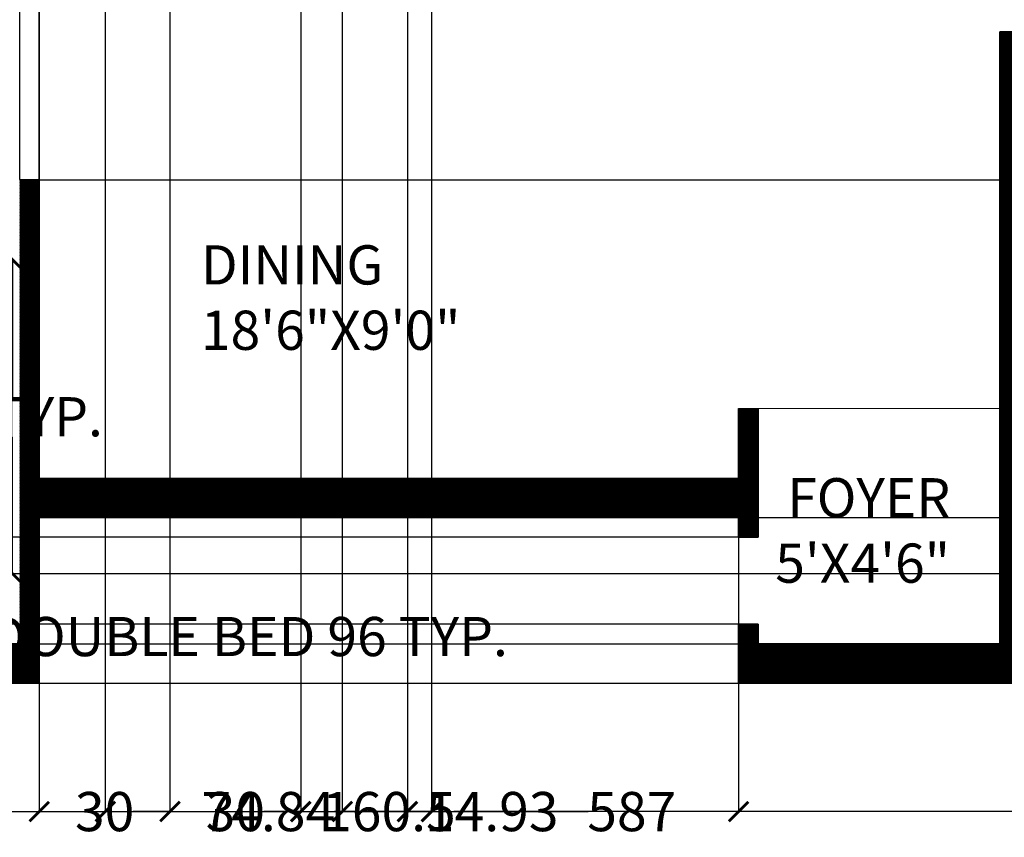
# Model space of a CAD drawing. Units: inches. Extents: x -9 to 675, y 146 to 566.
# Tile 2 of 4: x 192 to 418, y 146 to 334. Entities that reach past the tile are written whole.
import ezdxf

# ---------------------------------------------------------------- set-up
doc = ezdxf.new("R2010")
doc.units = ezdxf.units.IN
doc.header["$MEASUREMENT"] = 0
for name, color, linetype, lineweight in [('A-ANNO-DIMS', 2, 'Continuous', 18), ('A-AREA-IDEN', 7, 'Continuous', 18), ('A-FLOR-TRNS', 8, 'Continuous', 13), ('A-WALL', 7, 'Continuous', 35), ('A-WALL-PATT', 252, 'Continuous', 13)]:
    doc.layers.add(name, color=color, linetype=linetype, lineweight=lineweight)
doc.styles.get("Standard").update_dxf_attribs({"font": 'arial.ttf'})
doc.dimstyles.get("Standard").update_dxf_attribs({"dimtxt": 9, "dimasz": 4.5, "dimexe": 0.18, "dimexo": 0.0625, "dimgap": 0.09, "dimtad": 0, "dimtih": 1, "dimtoh": 1, "dimdec": 1, "dimzin": 0, "dimdsep": 46, "dimlunit": 4, "dimtxsty": 'Standard', "dimblk": 'ARCHTICK', "dimcen": 0.09, "dimadec": 0, "dimazin": 0, "dimtfac": 1, "dimtdec": 1, "dimtofl": 0, "dimtmove": 0, "dimatfit": 3, "dimfxl": 1, "dimtolj": 1, "dimtzin": 0, "dimarcsym": 0})

# ---------------------------------------------------------------- blocks, each defined once
blk = doc.blocks.new('_ArchTick')
at = {"color": 0, "linetype": 'ByBlock', "const_width": 0.15}
blk.add_lwpolyline([(-0.5, -0.5), (0.5, 0.5)], dxfattribs=at)
blk = doc.blocks.new('*D4')
at = {"layer": 'A-ANNO-DIMS', "color": 0, "lineweight": -2, "transparency": 16777216}
for p, q in [((80.28, 206.51), (80.28, 192)), ((176.28, 206.51), (176.28, 192)), ((80.28, 192.18), (176.28, 192.18)), ((176.28, 192.18), (180.78, 192.18))]:
    blk.add_line(p, q, dxfattribs=at)
at = {"layer": 'Defpoints', "color": 0, "transparency": 16777216}
for p in [(80.28, 206.58), (176.28, 206.58), (176.28, 192.18)]:
    blk.add_point(p, dxfattribs=at)
at = {"layer": 'A-ANNO-DIMS', "color": 0, "lineweight": -2, "transparency": 16777216, "xscale": 4.5, "yscale": 4.5, "zscale": 4.5, "rotation": 180}
blk.add_blockref('_ArchTick', (80.28, 192.18), dxfattribs=at)
at = {"layer": 'A-ANNO-DIMS', "color": 0, "lineweight": -2, "transparency": 16777216, "xscale": 4.5, "yscale": 4.5, "zscale": 4.5}
blk.add_blockref('_ArchTick', (176.28, 192.18), dxfattribs=at)
at = {"layer": 'A-ANNO-DIMS', "color": 0, "transparency": 16777216, "insert": (244.83, 192.18), "char_height": 9, "attachment_point": 5}
blk.add_mtext('\\A1;DOUBLE BED 96 TYP.', dxfattribs=at)
blk = doc.blocks.new('*D5')
at = {"layer": 'A-ANNO-DIMS', "color": 0, "lineweight": -2, "transparency": 16777216}
for p, q in [((176.35, 278.67), (190.86, 278.67)), ((190.68, 278.67), (190.68, 247.24)), ((190.68, 206.58), (190.68, 238.01)), ((176.35, 206.58), (190.86, 206.58))]:
    blk.add_line(p, q, dxfattribs=at)
at = {"layer": 'Defpoints', "color": 0, "transparency": 16777216}
for p in [(176.28, 278.67), (190.68, 278.67), (176.28, 206.58)]:
    blk.add_point(p, dxfattribs=at)
at = {"layer": 'A-ANNO-DIMS', "color": 0, "lineweight": -2, "transparency": 16777216, "xscale": 4.5, "yscale": 4.5, "zscale": 4.5}
for p, rotation in [((190.68, 278.67), 90), ((190.68, 206.58), 270)]:
    blk.add_blockref('_ArchTick', p, dxfattribs=dict(at, rotation=rotation))
at = {"layer": 'A-ANNO-DIMS', "color": 0, "transparency": 16777216, "insert": (190.68, 242.63), "char_height": 9, "attachment_point": 5}
blk.add_mtext('\\A1;72 TYP.', dxfattribs=at)
blk = doc.blocks.new('*D8')
at = {"layer": 'A-ANNO-DIMS', "color": 0, "lineweight": -2, "transparency": 16777216}
for p, q in [((626.3, 217.45), (626.3, 151.83)), ((39.3, 181.45), (39.3, 151.83)), ((39.3, 152.01), (322.77, 152.01)), ((626.3, 152.01), (342.83, 152.01))]:
    blk.add_line(p, q, dxfattribs=at)
at = {"layer": 'Defpoints', "color": 0, "transparency": 16777216}
for p in [(626.3, 217.51), (39.3, 181.51), (626.3, 152.01)]:
    blk.add_point(p, dxfattribs=at)
at = {"layer": 'A-ANNO-DIMS', "color": 0, "lineweight": -2, "transparency": 16777216, "xscale": 4.5, "yscale": 4.5, "zscale": 4.5, "rotation": 180}
blk.add_blockref('_ArchTick', (39.3, 152.01), dxfattribs=at)
at = {"layer": 'A-ANNO-DIMS', "color": 0, "lineweight": -2, "transparency": 16777216, "xscale": 4.5, "yscale": 4.5, "zscale": 4.5}
blk.add_blockref('_ArchTick', (626.3, 152.01), dxfattribs=at)
at = {"layer": 'A-ANNO-DIMS', "color": 0, "transparency": 16777216, "insert": (332.8, 152.01), "char_height": 9, "attachment_point": 5}
blk.add_mtext('\\A1;587', dxfattribs=at)
blk = doc.blocks.new('*D20')
at = {"layer": 'A-ANNO-DIMS', "color": 0, "lineweight": -2, "transparency": 16777216}
for p, q in [((196.8, 219.43), (196.8, 151.83)), ((357.3, 219.43), (357.3, 151.83)), ((196.8, 152.01), (262.17, 152.01)), ((357.3, 152.01), (291.94, 152.01))]:
    blk.add_line(p, q, dxfattribs=at)
at = {"layer": 'Defpoints', "color": 0, "transparency": 16777216}
for p in [(196.8, 219.49), (357.3, 219.49), (357.3, 152.01)]:
    blk.add_point(p, dxfattribs=at)
at = {"layer": 'A-ANNO-DIMS', "color": 0, "lineweight": -2, "transparency": 16777216, "xscale": 4.5, "yscale": 4.5, "zscale": 4.5, "rotation": 180}
blk.add_blockref('_ArchTick', (196.8, 152.01), dxfattribs=at)
at = {"layer": 'A-ANNO-DIMS', "color": 0, "lineweight": -2, "transparency": 16777216, "xscale": 4.5, "yscale": 4.5, "zscale": 4.5}
blk.add_blockref('_ArchTick', (357.3, 152.01), dxfattribs=at)
at = {"layer": 'A-ANNO-DIMS', "color": 0, "transparency": 16777216, "insert": (277.05, 152.01), "char_height": 9, "attachment_point": 5}
blk.add_mtext('\\A1;160.5', dxfattribs=at)
blk = doc.blocks.new('*D22')
at = {"layer": 'A-ANNO-DIMS', "color": 0, "lineweight": -2, "transparency": 16777216}
for p, q in [((196.87, 219.49), (655.98, 219.49)), ((655.8, 219.49), (655.8, 205.19)), ((655.8, 181.51), (655.8, 195.81)), ((196.87, 181.51), (655.98, 181.51))]:
    blk.add_line(p, q, dxfattribs=at)
at = {"layer": 'Defpoints', "color": 0, "transparency": 16777216}
for p in [(196.8, 219.49), (655.8, 219.49), (196.8, 181.51)]:
    blk.add_point(p, dxfattribs=at)
at = {"layer": 'A-ANNO-DIMS', "color": 0, "lineweight": -2, "transparency": 16777216, "xscale": 4.5, "yscale": 4.5, "zscale": 4.5}
for p, rotation in [((655.8, 219.49), 90), ((655.8, 181.51), 270)]:
    blk.add_blockref('_ArchTick', p, dxfattribs=dict(at, rotation=rotation))
at = {"layer": 'A-ANNO-DIMS', "color": 0, "transparency": 16777216, "insert": (655.8, 200.5), "char_height": 9, "attachment_point": 5}
blk.add_mtext('\\A1;37.98', dxfattribs=at)
blk = doc.blocks.new('*D26')
at = {"layer": 'A-ANNO-DIMS', "color": 0, "lineweight": -2, "transparency": 16777216}
for p, q in [((211.96, 521.95), (211.96, 151.83)), ((286.8, 521.95), (286.8, 151.83)), ((211.96, 152.01), (234.16, 152.01)), ((286.8, 152.01), (264.6, 152.01))]:
    blk.add_line(p, q, dxfattribs=at)
at = {"layer": 'Defpoints', "color": 0, "transparency": 16777216}
for p in [(211.96, 522.01), (286.8, 522.01), (286.8, 152.01)]:
    blk.add_point(p, dxfattribs=at)
at = {"layer": 'A-ANNO-DIMS', "color": 0, "lineweight": -2, "transparency": 16777216, "xscale": 4.5, "yscale": 4.5, "zscale": 4.5, "rotation": 180}
blk.add_blockref('_ArchTick', (211.96, 152.01), dxfattribs=at)
at = {"layer": 'A-ANNO-DIMS', "color": 0, "lineweight": -2, "transparency": 16777216, "xscale": 4.5, "yscale": 4.5, "zscale": 4.5}
blk.add_blockref('_ArchTick', (286.8, 152.01), dxfattribs=at)
at = {"layer": 'A-ANNO-DIMS', "color": 0, "transparency": 16777216, "insert": (249.38, 152.01), "char_height": 9, "attachment_point": 5}
blk.add_mtext('\\A1;74.84', dxfattribs=at)
blk = doc.blocks.new('*D28')
at = {"layer": 'A-ANNO-DIMS', "color": 0, "lineweight": -2, "transparency": 16777216}
for p, q in [((196.8, 469.45), (196.8, 151.83)), ((226.8, 469.45), (226.8, 151.83)), ((196.8, 152.01), (205.28, 152.01)), ((226.8, 152.01), (218.32, 152.01))]:
    blk.add_line(p, q, dxfattribs=at)
at = {"layer": 'Defpoints', "color": 0, "transparency": 16777216}
for p in [(196.8, 469.51), (226.8, 469.51), (226.8, 152.01)]:
    blk.add_point(p, dxfattribs=at)
at = {"layer": 'A-ANNO-DIMS', "color": 0, "lineweight": -2, "transparency": 16777216, "xscale": 4.5, "yscale": 4.5, "zscale": 4.5, "rotation": 180}
blk.add_blockref('_ArchTick', (196.8, 152.01), dxfattribs=at)
at = {"layer": 'A-ANNO-DIMS', "color": 0, "lineweight": -2, "transparency": 16777216, "xscale": 4.5, "yscale": 4.5, "zscale": 4.5}
blk.add_blockref('_ArchTick', (226.8, 152.01), dxfattribs=at)
at = {"layer": 'A-ANNO-DIMS', "color": 0, "transparency": 16777216, "insert": (211.8, 152.01), "char_height": 9, "attachment_point": 5}
blk.add_mtext('\\A1;30', dxfattribs=at)
blk = doc.blocks.new('*D29')
at = {"layer": 'A-ANNO-DIMS', "color": 0, "lineweight": -2, "transparency": 16777216}
for p, q in [((226.8, 469.45), (226.8, 151.83)), ((256.8, 469.45), (256.8, 151.83)), ((226.8, 152.01), (235.28, 152.01)), ((256.8, 152.01), (248.32, 152.01))]:
    blk.add_line(p, q, dxfattribs=at)
at = {"layer": 'Defpoints', "color": 0, "transparency": 16777216}
for p in [(226.8, 469.51), (256.8, 469.51), (256.8, 152.01)]:
    blk.add_point(p, dxfattribs=at)
at = {"layer": 'A-ANNO-DIMS', "color": 0, "lineweight": -2, "transparency": 16777216, "xscale": 4.5, "yscale": 4.5, "zscale": 4.5, "rotation": 180}
blk.add_blockref('_ArchTick', (226.8, 152.01), dxfattribs=at)
at = {"layer": 'A-ANNO-DIMS', "color": 0, "lineweight": -2, "transparency": 16777216, "xscale": 4.5, "yscale": 4.5, "zscale": 4.5}
blk.add_blockref('_ArchTick', (256.8, 152.01), dxfattribs=at)
at = {"layer": 'A-ANNO-DIMS', "color": 0, "transparency": 16777216, "insert": (241.8, 152.01), "char_height": 9, "attachment_point": 5}
blk.add_mtext('\\A1;30', dxfattribs=at)
blk = doc.blocks.new('*D30')
at = {"layer": 'A-ANNO-DIMS', "color": 0, "lineweight": -2, "transparency": 16777216}
for p, q in [((226.8, 347.95), (226.8, 151.83)), ((256.8, 347.95), (256.8, 151.83)), ((226.8, 152.01), (235.28, 152.01)), ((256.8, 152.01), (248.32, 152.01))]:
    blk.add_line(p, q, dxfattribs=at)
at = {"layer": 'Defpoints', "color": 0, "transparency": 16777216}
for p in [(226.8, 348.01), (256.8, 348.01), (256.8, 152.01)]:
    blk.add_point(p, dxfattribs=at)
at = {"layer": 'A-ANNO-DIMS', "color": 0, "lineweight": -2, "transparency": 16777216, "xscale": 4.5, "yscale": 4.5, "zscale": 4.5, "rotation": 180}
blk.add_blockref('_ArchTick', (226.8, 152.01), dxfattribs=at)
at = {"layer": 'A-ANNO-DIMS', "color": 0, "lineweight": -2, "transparency": 16777216, "xscale": 4.5, "yscale": 4.5, "zscale": 4.5}
blk.add_blockref('_ArchTick', (256.8, 152.01), dxfattribs=at)
at = {"layer": 'A-ANNO-DIMS', "color": 0, "transparency": 16777216, "insert": (241.8, 152.01), "char_height": 9, "attachment_point": 5}
blk.add_mtext('\\A1;30', dxfattribs=at)
blk = doc.blocks.new('*D34')
at = {"layer": 'A-ANNO-DIMS', "color": 0, "lineweight": -2, "transparency": 16777216}
for p, q in [((196.87, 339.01), (655.98, 339.01)), ((655.8, 339.01), (655.8, 322.62)), ((655.8, 297.01), (655.8, 313.4)), ((196.87, 297.01), (655.98, 297.01))]:
    blk.add_line(p, q, dxfattribs=at)
at = {"layer": 'Defpoints', "color": 0, "transparency": 16777216}
for p in [(196.8, 339.01), (655.8, 339.01), (196.8, 297.01)]:
    blk.add_point(p, dxfattribs=at)
at = {"layer": 'A-ANNO-DIMS', "color": 0, "lineweight": -2, "transparency": 16777216, "xscale": 4.5, "yscale": 4.5, "zscale": 4.5}
for p, rotation in [((655.8, 339.01), 90), ((655.8, 297.01), 270)]:
    blk.add_blockref('_ArchTick', p, dxfattribs=dict(at, rotation=rotation))
at = {"layer": 'A-ANNO-DIMS', "color": 0, "transparency": 16777216, "insert": (655.8, 318.01), "char_height": 9, "attachment_point": 5}
blk.add_mtext('\\A1;42', dxfattribs=at)
blk = doc.blocks.new('*D39')
at = {"layer": 'A-ANNO-DIMS', "color": 0, "lineweight": -2, "transparency": 16777216}
for p, q in [((357.24, 214.99), (9.62, 214.99)), ((9.8, 214.99), (9.8, 209.69)), ((9.8, 195.01), (9.8, 200.32)), ((357.24, 195.01), (9.62, 195.01))]:
    blk.add_line(p, q, dxfattribs=at)
at = {"layer": 'Defpoints', "color": 0, "transparency": 16777216}
for p in [(9.8, 214.99), (357.3, 214.99), (357.3, 195.01)]:
    blk.add_point(p, dxfattribs=at)
at = {"layer": 'A-ANNO-DIMS', "color": 0, "lineweight": -2, "transparency": 16777216, "xscale": 4.5, "yscale": 4.5, "zscale": 4.5}
for p, rotation in [((9.8, 214.99), 90), ((9.8, 195.01), 270)]:
    blk.add_blockref('_ArchTick', p, dxfattribs=dict(at, rotation=rotation))
at = {"layer": 'A-ANNO-DIMS', "color": 0, "transparency": 16777216, "insert": (9.8, 205), "char_height": 9, "attachment_point": 5}
blk.add_mtext('\\A1;19.98', dxfattribs=at)
blk = doc.blocks.new('*D45')
at = {"layer": 'A-ANNO-DIMS', "color": 0, "lineweight": -2, "transparency": 16777216}
for p, q in [((80.35, 206.67), (655.98, 206.67)), ((655.8, 206.67), (655.8, 203.28)), ((655.8, 190.51), (655.8, 193.91)), ((48.37, 190.51), (655.98, 190.51))]:
    blk.add_line(p, q, dxfattribs=at)
at = {"layer": 'Defpoints', "color": 0, "transparency": 16777216}
for p in [(80.28, 206.67), (655.8, 206.67), (48.3, 190.51)]:
    blk.add_point(p, dxfattribs=at)
at = {"layer": 'A-ANNO-DIMS', "color": 0, "lineweight": -2, "transparency": 16777216, "xscale": 4.5, "yscale": 4.5, "zscale": 4.5}
for p, rotation in [((655.8, 206.67), 90), ((655.8, 190.51), 270)]:
    blk.add_blockref('_ArchTick', p, dxfattribs=dict(at, rotation=rotation))
at = {"layer": 'A-ANNO-DIMS', "color": 0, "transparency": 16777216, "insert": (655.8, 198.59), "char_height": 9, "attachment_point": 5}
blk.add_mtext('\\A1;16.165', dxfattribs=at)
blk = doc.blocks.new('*D50')
at = {"layer": 'A-ANNO-DIMS', "color": 0, "lineweight": -2, "transparency": 16777216}
for p, q in [((192.3, 297.07), (192.3, 560.69)), ((192.3, 560.51), (196.8, 560.51)), ((196.8, 297.07), (196.8, 560.69)), ((196.8, 560.51), (201.3, 560.51))]:
    blk.add_line(p, q, dxfattribs=at)
at = {"layer": 'Defpoints', "color": 0, "transparency": 16777216}
for p in [(196.8, 560.51), (192.3, 297.01), (196.8, 297.01)]:
    blk.add_point(p, dxfattribs=at)
at = {"layer": 'A-ANNO-DIMS', "color": 0, "lineweight": -2, "transparency": 16777216, "xscale": 4.5, "yscale": 4.5, "zscale": 4.5, "rotation": 180}
blk.add_blockref('_ArchTick', (192.3, 560.51), dxfattribs=at)
at = {"layer": 'A-ANNO-DIMS', "color": 0, "lineweight": -2, "transparency": 16777216, "xscale": 4.5, "yscale": 4.5, "zscale": 4.5}
blk.add_blockref('_ArchTick', (196.8, 560.51), dxfattribs=at)
at = {"layer": 'A-ANNO-DIMS', "color": 0, "transparency": 16777216, "insert": (209.8, 560.51), "char_height": 9, "attachment_point": 5}
blk.add_mtext('\\A1;4.5', dxfattribs=at)
blk = doc.blocks.new('*D51')
at = {"layer": 'A-ANNO-DIMS', "color": 0, "lineweight": -2, "transparency": 16777216}
for p, q in [((266.36, 416.64), (266.36, 151.83)), ((281.29, 416.64), (281.29, 151.83)), ((266.36, 152.01), (281.29, 152.01)), ((281.29, 152.01), (285.79, 152.01))]:
    blk.add_line(p, q, dxfattribs=at)
at = {"layer": 'Defpoints', "color": 0, "transparency": 16777216}
for p in [(266.36, 416.7), (281.29, 416.7), (281.29, 152.01)]:
    blk.add_point(p, dxfattribs=at)
at = {"layer": 'A-ANNO-DIMS', "color": 0, "lineweight": -2, "transparency": 16777216, "xscale": 4.5, "yscale": 4.5, "zscale": 4.5, "rotation": 180}
blk.add_blockref('_ArchTick', (266.36, 152.01), dxfattribs=at)
at = {"layer": 'A-ANNO-DIMS', "color": 0, "lineweight": -2, "transparency": 16777216, "xscale": 4.5, "yscale": 4.5, "zscale": 4.5}
blk.add_blockref('_ArchTick', (281.29, 152.01), dxfattribs=at)
at = {"layer": 'A-ANNO-DIMS', "color": 0, "transparency": 16777216, "insert": (300.65, 152.01), "char_height": 9, "attachment_point": 5}
blk.add_mtext('\\A1;14.93', dxfattribs=at)

msp = doc.modelspace()

# ---------------------------------------------------------------- hatches: boundary and pattern name
at = {"layer": 'A-WALL-PATT'}
h = msp.add_hatch(dxfattribs=at)
h.set_pattern_fill('ANSI31', color=256)
h.paths.add_polyline_path([(361.8026, 244.5097), (357.3026, 244.5097), (357.3026, 228.4917), (286.8026, 228.4917), (196.8026, 228.4917), (196.8026, 297.0097), (192.3026, 297.0097), (192.3026, 190.5097), (196.8026, 190.5097), (196.8026, 219.4917), (286.8026, 219.4917), (357.3026, 219.4917), (357.3026, 217.5097), (357.3026, 214.9917), (361.8026, 214.9917), (361.8026, 217.5097)])
h.paths.add_polyline_path([(532.6092, 217.5097), (541.8026, 217.5097), (550.8026, 217.5097), (626.3026, 217.5097), (626.3026, 373.5097), (626.3026, 378.0097), (617.3026, 378.0097), (617.3026, 373.5097), (617.3026, 226.5097), (550.8026, 226.5097), (541.8026, 226.5097), (488.3026, 226.5097), (488.3026, 331.0097), (483.8026, 331.0097), (474.8026, 331.0097), (474.8026, 326.5097), (483.8026, 326.5097), (483.8026, 226.5097), (421.8026, 226.5097), (421.8026, 326.5097), (444.8026, 326.5097), (444.8026, 331.0097), (421.8026, 331.0097), (417.3026, 331.0097), (417.3026, 217.5097), (417.3026, 190.5097), (387.6027, 190.5097), (361.8026, 190.5097), (361.8026, 195.0097), (357.3026, 195.0097), (357.3026, 190.5097), (357.3026, 181.5097), (387.6027, 181.5097), (421.8026, 181.5097), (532.6092, 181.5097)])
h.paths.add_polyline_path([(421.8026, 190.5097), (421.8026, 217.5097), (523.6092, 217.5097), (523.6092, 190.5097)], flags=16)
h.paths.add_polyline_path([(550.8026, 378.0097), (550.8026, 531.0097), (525.3955, 531.0097), (525.3955, 522.0097), (541.8026, 522.0097), (541.8026, 378.0097), (472.8026, 378.0097), (472.8026, 373.5097), (483.8026, 373.5097), (488.3026, 373.5097), (541.8026, 373.5097), (550.8026, 373.5097)])
h.paths.add_polyline_path([(130.3026, 469.5097), (146.3026, 469.5097), (146.3026, 474.0097), (130.3026, 474.0097), (130.3026, 522.0097), (143.3026, 522.0097), (143.3026, 531.0097), (121.3026, 531.0097), (121.3026, 351.7597), (121.3026, 348.0097), (130.3026, 348.0097), (139.3026, 348.0097), (139.3026, 351.7597), (130.3026, 351.7597)])
h.paths.add_polyline_path([(211.9624, 531.0097), (179.3026, 531.0097), (179.3026, 522.0097), (192.3026, 522.0097), (192.3026, 474.0097), (176.3026, 474.0097), (176.3026, 469.5097), (192.3026, 469.5097), (192.3026, 351.7597), (169.3026, 351.7597), (169.3026, 348.0097), (192.3026, 348.0097), (192.3026, 339.0097), (196.8026, 339.0097), (196.8026, 348.0097), (226.8026, 348.0097), (226.8026, 352.5097), (196.8026, 352.5097), (196.8026, 469.5097), (226.8026, 469.5097), (226.8026, 474.0097), (196.8026, 474.0097), (196.8026, 522.0097), (211.9624, 522.0097)])
h.paths.add_polyline_path([(291.3026, 522.0097), (291.3026, 531.0097), (286.8026, 531.0097), (286.8026, 522.0097), (286.8026, 352.5097), (256.8026, 352.5097), (256.8026, 348.0097), (286.8026, 348.0097), (286.8026, 346.5097), (291.3026, 346.5097)])
h.paths.add_polyline_path([(417.3026, 474.0097), (291.3026, 474.0097), (291.3026, 469.5097), (417.3026, 469.5097)])
h.paths.add_polyline_path([(421.8026, 522.0097), (435.8002, 522.0097), (435.8002, 531.0097), (417.3026, 531.0097), (417.3026, 522.0097), (417.3026, 373.5097), (421.8026, 373.5097), (430.8026, 373.5097), (430.8026, 378.0097), (421.8026, 378.0097)])
h.paths.add_polyline_path([(48.3026, 348.0097), (48.3026, 351.7597), (39.3026, 351.7597), (39.3026, 348.0097), (39.3026, 181.5097), (121.3026, 181.5097), (196.8026, 181.5097), (196.8026, 190.5097), (192.3026, 190.5097), (121.3026, 190.5097), (48.3026, 190.5097)])

# ---------------------------------------------------------------- linework, layer by layer
at = {"layer": 'A-FLOR-TRNS'}
for q in [(357.3026, 244.5097), (417.3026, 244.5097)]:
    msp.add_line((387.6027, 244.5097), q, dxfattribs=at)
at = {"layer": 'A-WALL'}
for p, q in [((421.8026, 331.0097), (417.3026, 331.0097)), ((417.3026, 331.0097), (417.3026, 217.5097)), ((192.3026, 297.0097), (196.8026, 297.0097)), ((196.8026, 297.0097), (196.8026, 228.4917)), ((357.3026, 244.5097), (357.3026, 228.4917)), ((361.8026, 244.5097), (361.8026, 217.5097)), ((286.8026, 228.4917), (196.8026, 228.4917)), ((286.8026, 228.4917), (357.3026, 228.4917)), ((286.8026, 219.4917), (196.8026, 219.4917)), ((196.8026, 219.4917), (196.8026, 190.5097)), ((286.8026, 219.4917), (357.3026, 219.4917)), ((357.3026, 219.4917), (357.3026, 217.5097)), ((357.3026, 217.5097), (357.3026, 214.9917)), ((361.8026, 217.5097), (361.8026, 214.9917)), ((417.3026, 217.5097), (417.3026, 190.5097)), ((357.3026, 214.9917), (361.8026, 214.9917)), ((361.8026, 195.0097), (357.3026, 195.0097)), ((357.3026, 195.0097), (357.3026, 190.5097)), ((361.8026, 195.0097), (361.8026, 190.5097)), ((196.8026, 190.5097), (121.3026, 190.5097)), ((196.8026, 190.5097), (196.8026, 181.5097)), ((357.3026, 190.5097), (357.3026, 181.5097)), ((387.6027, 190.5097), (361.8026, 190.5097)), ((387.6027, 190.5097), (417.3026, 190.5097)), ((196.8026, 181.5097), (121.3026, 181.5097)), ((387.6027, 181.5097), (357.3026, 181.5097)), ((421.8026, 181.5097), (387.6027, 181.5097))]:
    msp.add_line(p, q, dxfattribs=at)

# ---------------------------------------------------------------- texts
at = {"layer": 'A-AREA-IDEN', "char_height": 9, "attachment_point": 1}
for s, insert in [('DINING\\P18\'6"X9\'0"', (233.8964, 281.9888)), ('   FOYER\\P  5\'X4\'6"', (360.2278, 228.5369))]:
    msp.add_mtext_dynamic_manual_height_columns(s, width=552.217276, gutter_width=1, heights=[0], dxfattribs=dict(at, insert=insert))

# ---------------------------------------------------------------- dimensions: what is measured, and where the dimension line sits
at = {"layer": 'A-ANNO-DIMS'}
for base, p1, p2, override, picture, middle in [((196.8026, 560.5097), (192.3026, 297.0097), (196.8026, 297.0097), {"dimdec": 1, "dimlfac": 1, "dimrnd": 0, "dimzin": 0, "dimdsep": 46, "dimlunit": 2}, '*D50', (209.8002, 560.5097)), ((286.8026, 152.0097), (211.9624, 522.0097), (286.8026, 522.0097), {"dimdec": 2, "dimlfac": 1, "dimrnd": 0, "dimzin": 0, "dimdsep": 46, "dimlunit": 2}, '*D26', (249.3825, 152.0097)), ((226.8026, 152.0097), (196.8026, 469.5097), (226.8026, 469.5097), {"dimdec": 0, "dimlfac": 1, "dimrnd": 0, "dimzin": 0, "dimdsep": 46, "dimlunit": 2}, '*D28', (211.8026, 152.0097)), ((256.8026, 152.0097), (226.8026, 469.5097), (256.8026, 469.5097), {"dimdec": 0, "dimlfac": 1, "dimrnd": 0, "dimzin": 0, "dimdsep": 46, "dimlunit": 2}, '*D29', (241.8026, 152.0097)), ((281.2941, 152.0097), (266.363, 416.6988), (281.2941, 416.6988), {"dimdec": 2, "dimlfac": 1, "dimrnd": 0, "dimzin": 0, "dimdsep": 46, "dimlunit": 2}, '*D51', (300.6457, 152.0097)), ((256.8026, 152.0097), (226.8026, 348.0097), (256.8026, 348.0097), {"dimdec": 0, "dimlfac": 1, "dimrnd": 0, "dimzin": 0, "dimdsep": 46, "dimlunit": 2}, '*D30', (241.8026, 152.0097)), ((357.3026, 152.0097), (196.8026, 219.4917), (357.3026, 219.4917), {"dimdec": 1, "dimlfac": 1, "dimrnd": 0, "dimzin": 0, "dimdsep": 46, "dimlunit": 2}, '*D20', (277.0526, 152.0097)), ((626.3026, 152.0097), (39.3026, 181.5097), (626.3026, 217.5097), {"dimdec": 0, "dimlfac": 1, "dimrnd": 0, "dimzin": 0, "dimdsep": 46, "dimlunit": 2}, '*D8', (332.8026, 152.0097))]:
    dim = msp.add_linear_dim(base=base, p1=p1, p2=p2, dimstyle='Standard', override=override, dxfattribs=at)
    dim.commit()
    dim.dimension.update_dxf_attribs({"geometry": picture, "text_midpoint": middle})
for base, p1, p2, override, picture, middle in [((655.8026, 339.0097), (196.8026, 297.0097), (196.8026, 339.0097), {"dimdec": 0, "dimlfac": 1, "dimrnd": 0, "dimzin": 0, "dimdsep": 46, "dimlunit": 2}, '*D34', (655.8026, 318.0097)), ((655.8026, 219.4917), (196.8026, 181.5097), (196.8026, 219.4917), {"dimdec": 2, "dimlfac": 1, "dimrnd": 0, "dimzin": 0, "dimdsep": 46, "dimlunit": 2}, '*D22', (655.8026, 200.5007)), ((9.8026, 214.9917), (357.3026, 195.0097), (357.3026, 214.9917), {"dimdec": 2, "dimlfac": 1, "dimrnd": 0, "dimzin": 0, "dimdsep": 46, "dimlunit": 2}, '*D39', (9.8026, 205.0007)), ((655.8026, 206.6747), (48.3026, 190.5097), (80.2837, 206.6747), {"dimdec": 3, "dimlfac": 1, "dimrnd": 0, "dimzin": 0, "dimdsep": 46, "dimlunit": 2}, '*D45', (655.8026, 198.5922))]:
    dim = msp.add_linear_dim(base=base, p1=p1, p2=p2, angle=90, dimstyle='Standard', override=override, dxfattribs=at)
    dim.commit()
    dim.dimension.update_dxf_attribs({"geometry": picture, "text_midpoint": middle})
dim = msp.add_linear_dim(base=(190.6837, 278.6747), p1=(176.2837, 206.5772), p2=(176.2837, 278.6747), angle=90, text='<> TYP.', dimstyle='Standard', override={"dimdec": 0, "dimlfac": 1, "dimrnd": 0, "dimzin": 0, "dimdsep": 46, "dimlunit": 2}, dxfattribs=at)
dim.commit()
dim.dimension.update_dxf_attribs({"geometry": '*D5', "text_midpoint": (190.6837, 242.6259)})
dim = msp.add_linear_dim(base=(176.2837, 192.1772), p1=(80.2837, 206.5772), p2=(176.2837, 206.5772), text='DOUBLE BED <> TYP.', dimstyle='Standard', override={"dimdec": 0, "dimlfac": 1, "dimrnd": 0, "dimzin": 0, "dimdsep": 46, "dimlunit": 2}, dxfattribs=at)
dim.commit()
dim.dimension.update_dxf_attribs({"geometry": '*D4', "text_midpoint": (244.8253, 192.1772)})

doc.saveas('drawing.dxf')
